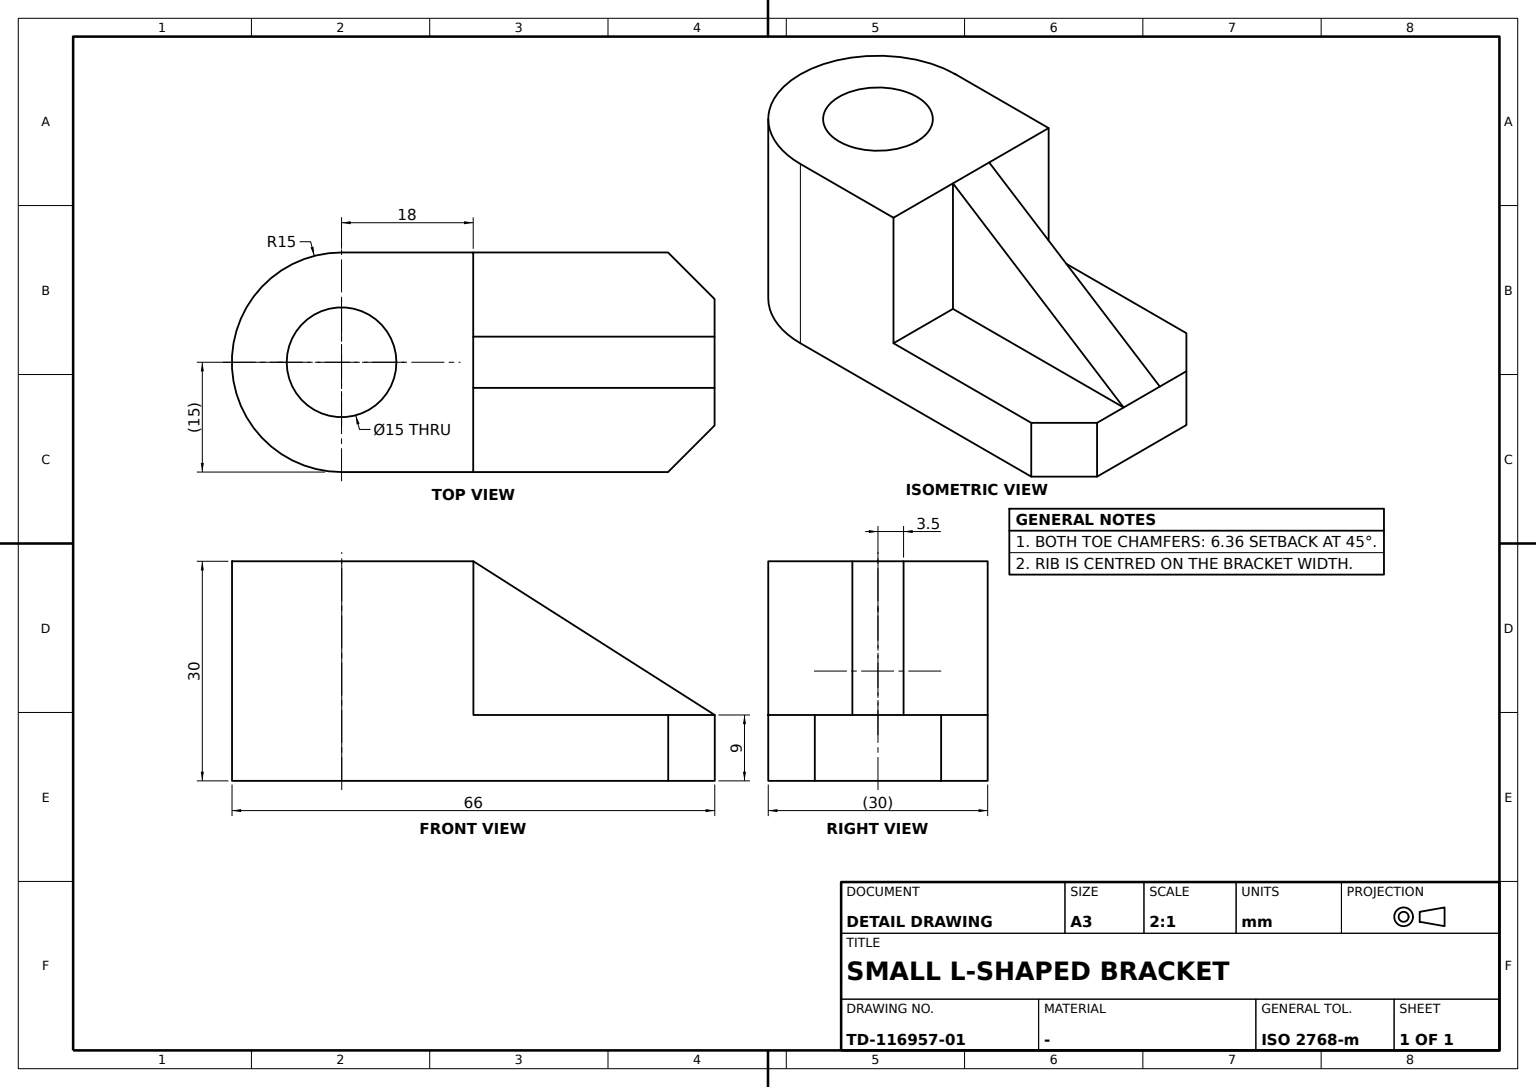
CATIA V5 part; units mm, degrees
sketch "Sketch1" plane through (0, 0, 0) normal (0, 0, 1) x (1, 0, 0)
  line L0 (0, 15) -> (-18, 15)
  line L1 (-18, -15) -> (0, -15)
  line L2 (0, -15) -> (0, 15)
  arc A0 (-18, 15) -> (-18, -15) centre (-18, 0) ccw
  circle A1 centre (-18, 0) radius 7.5
  dimension "length L2" = 30
  dimension "length L0" = 18
  dimension "radius A0" = 15
  dimension "distance L2 y axis" = 0
  dimension "radius A1" = 7.5
  constraint horizontal L0 x-axis
  constraint horizontal L1 x-axis
  constraint vertical L2 y-axis
  constraint symmetry L0 L1 x-axis
  constraint tangency A0 L0
extrude "Pad1" add sketch "Sketch1" along normal blind 30
sketch "Sketch2" plane through (0, 0, 0) normal (0, 0, 1) x (1, 0, 0)
  line L0 (0, 15) -> (26.636, 15)
  line L1 (33, 8.636) -> (33, -8.636)
  line L2 (26.636, -15) -> (0, -15)
  line L3 (0, -15) -> (0, 15)
  point P0 (33, 15)
  point P1 (33, -15)
  line L4 (26.636, 15) -> (33, 8.636)
  line L5 (33, -8.636) -> (26.636, -15)
  dimension "distance y axis L3" = 0
  dimension "angle L0 L4" = 45
  dimension "length L4" = 9
  dimension "angle L1 L5" = 45
  dimension "length L5" = 9
  dimension "distance y axis L1" = 33
  dimension "distance L2 L0" = 30
  constraint horizontal L0 x-axis
  constraint horizontal L2 x-axis
  constraint vertical L1 y-axis
  constraint vertical L3 y-axis
  constraint symmetry L0 L2 x-axis
extrude "Pad2" add sketch "Sketch2" along normal blind 9
sketch "Sketch3" plane through (0, 0, 0) normal (0, 1, 0) x (-1, 0, 0)
  point P0 (0, 30)
  line L0 (0, 30) -> (0, 9)
  line L1 (0, 9) -> (-33, 9)
  point P1 (-33, 9)
  line L2 (-33, 9) -> (0, 30)
  line L3 (-26.636, 9) -> (0, 9) construction
  point P2 (0, 30)
  point P3 (-33, 9)
  constraint vertical L0 y-axis
  constraint horizontal L1 x-axis
  constraint coincidence L1 L3
  constraint coincidence P0 P2
  constraint coincidence P1 P3
extrude "Pad3" add sketch "Sketch3" along normal mid plane 7
properties part number "1"
